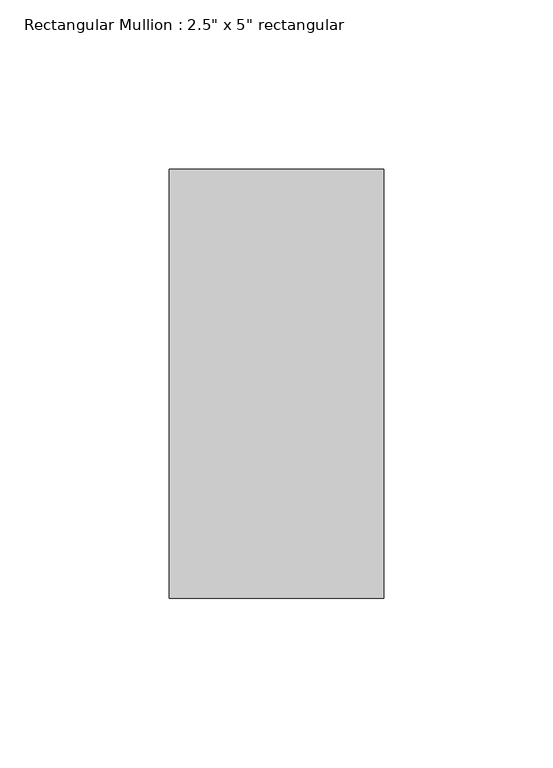
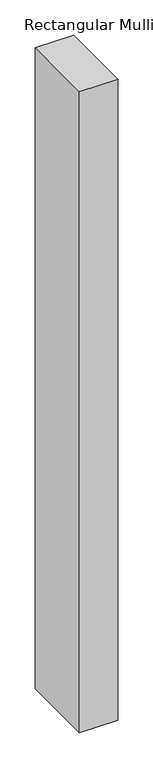
"""IFC4 building model written with IfcOpenShell, lengths in millimetres: member geometry."""

from ifc_helpers import new_model, si_unit, frame, origin, place, context, project, spatial, polyline, outline, extrude, source, transform, mapped, element, save


def member_b546c93c(model_context):
    return source(origin(), model_context, "Body", "SweptSolid", [
        extrude(outline(polyline([(31.75, 63.5), (31.75, -63.5), (-31.75, -63.5), (-31.75, 63.5), (31.75, 63.5)])), frame((0.0, 0.0, -1117.6), z_axis=(0.0, 0.0, 1.0), x_axis=(1.0, 0.0, 0.0)), (0.0, 0.0, 1.0), 1117.6),
    ])


if __name__ == "__main__":
    model = new_model("IFC4")
    model_context = context("Model", 3, world=origin())
    ifc_project = project(units=[si_unit("LENGTHUNIT", "METRE", prefix="MILLI")], contexts=[model_context])
    site = spatial("IfcSite", under=ifc_project)
    building = spatial("IfcBuilding", under=site)
    placement = place(None, origin())
    member_shape = member_b546c93c(model_context)
    element("IfcMember", 1, ObjectType="Rectangular Mullion : 2.5\" x 5\" rectangular", at=placement, inside=building, context=model_context, shape_type="MappedRepresentation", body=[
        mapped(member_shape, transform((0.0, 0.0, 0.0), x_axis=(1.0, 0.0, 0.0), y_axis=(0.0, 1.0, 0.0), z_axis=(0.0, 0.0, 1.0))),
    ])
    save(model, "model.ifc")

# Revit data of these elements
# Type "Rectangular Mullion : 2.5\" x 5\" rectangular"
#   built-in parameter 1007304 = 0.416667 (stored number, unit not read)
#   built-in parameter 1007301 = 0.104167 (stored number, unit not read)
#   built-in parameter 1007300 = 0.104167 (stored number, unit not read)
# Element 1 (IfcMember, "Rectangular Mullion : 2.5\" x 5\" rectangular")
#   Materials on its faces: "Aluminum"
# Materials
#   "Aluminum": class "Metal", colour RGB 247 247 247, transparency 0, Description = "Aluminum 6061", Cost = 0
